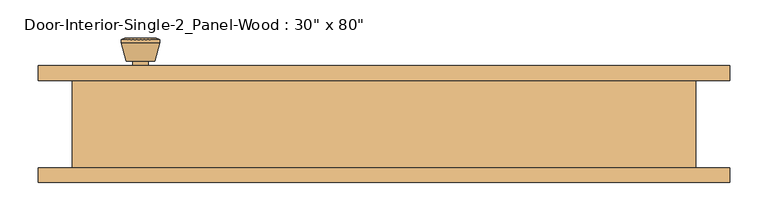
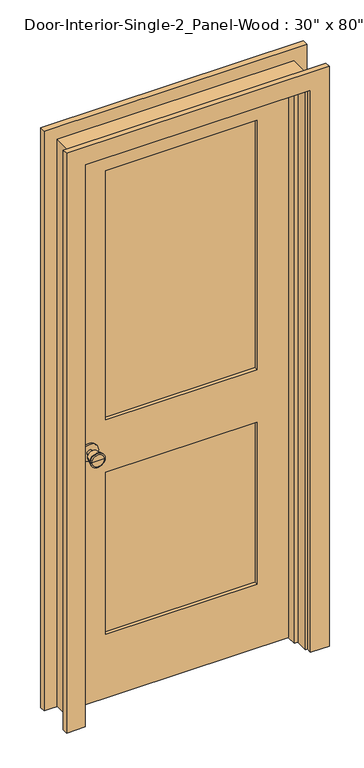
"""IFC4 building model written with IfcOpenShell, lengths in millimetres: door geometry."""

from ifc_helpers import new_model, si_unit, point, frame, frame_2d, origin, place, context, project, spatial, polyline, circle_curve, trimmed, segment, composite_curve, outline, extrude, faceted_brep, source, transform, mapped, element, save
from ifc_brep_helpers import plane_surface, cylinder_surface, revolved_surface, advanced_brep


def door_45c5d68b(model_context):
    return source(origin(), model_context, "Body", "SolidModel", [
        advanced_brep(
        [(-317.5, 13.05, 914.4), (-307.5, 13.05, 914.4), (-327.5, 13.05, 914.4), (-297.0241324, -35.95, 914.4), (-317.5, -35.95, 914.4), (-337.9758676, -35.95, 914.4), (-292.5, -34.1221319, 914.4), (-342.5, -34.1221319, 914.4), (-292.5, -30.6584537, 914.4), (-342.5, -30.6584537, 914.4), (-298.863764, -5.95, 914.4), (-336.136236, -5.95, 914.4), (-307.5, -5.95, 914.4), (-327.5, -5.95, 914.4)],
        [
            (0, 1),
            (1, 2, circle_curve(frame((-317.5, 13.05, 914.4), z_axis=(0.0, 1.0, 0.0), x_axis=(-1.0, 0.0, 0.0)), 10.0)),
            (2, 0),
            (2, 1, circle_curve(frame((-317.5, 13.05, 914.4), z_axis=(0.0, 1.0, 0.0), x_axis=(-1.0, 0.0, 0.0)), 10.0)),
            (3, 4),
            (4, 5),
            (5, 3, circle_curve(frame((-317.5, -35.95, 914.4), z_axis=(0.0, -1.0, 0.0), x_axis=(-1.0, 0.0, 0.0)), 20.4758676)),
            (3, 5, circle_curve(frame((-317.5, -35.95, 914.4), z_axis=(0.0, -1.0, 0.0), x_axis=(-1.0, 0.0, 0.0)), 20.4758676)),
            (6, 3),
            (5, 7),
            (7, 6, circle_curve(frame((-317.5, -34.1221319, 914.4), z_axis=(0.0, -1.0, 0.0), x_axis=(-1.0, 0.0, 0.0)), 25.0)),
            (6, 7, circle_curve(frame((-317.5, -34.1221319, 914.4), z_axis=(0.0, -1.0, 0.0), x_axis=(-1.0, 0.0, 0.0)), 25.0)),
            (8, 6),
            (7, 9),
            (9, 8, circle_curve(frame((-317.5, -30.6584537, 914.4), z_axis=(0.0, -1.0, 0.0), x_axis=(-1.0, 0.0, 0.0)), 25.0)),
            (8, 9, circle_curve(frame((-317.5, -30.6584537, 914.4), z_axis=(0.0, -1.0, 0.0), x_axis=(-1.0, 0.0, 0.0)), 25.0)),
            (10, 8),
            (9, 11),
            (11, 10, circle_curve(frame((-317.5, -5.95, 914.4), z_axis=(0.0, -1.0, 0.0), x_axis=(-1.0, 0.0, 0.0)), 18.636236)),
            (10, 11, circle_curve(frame((-317.5, -5.95, 914.4), z_axis=(0.0, -1.0, 0.0), x_axis=(-1.0, 0.0, 0.0)), 18.636236)),
            (12, 10),
            (11, 13),
            (13, 12, circle_curve(frame((-317.5, -5.95, 914.4), z_axis=(0.0, -1.0, 0.0), x_axis=(-1.0, 0.0, 0.0)), 10.0)),
            (12, 13, circle_curve(frame((-317.5, -5.95, 914.4), z_axis=(0.0, -1.0, 0.0), x_axis=(-1.0, 0.0, 0.0)), 10.0)),
            (1, 12),
            (13, 2),
        ],
        [
            plane_surface(frame((-317.5, 13.05, 914.4), z_axis=(0.0, 1.0, 0.0), x_axis=(-1.0, 0.0, 0.0))),
            plane_surface(frame((-317.5, -35.95, 914.4), z_axis=(0.0, -1.0, 0.0), x_axis=(-1.0, 0.0, 0.0))),
            revolved_surface(polyline([(-337.9758676, -35.95, 914.4), (-342.5, -34.1221319, 914.4)]), (-317.5, 13.05, 914.4), (0.0, 1.0, 0.0)),
            cylinder_surface(frame((-317.5, 13.05, 914.4), z_axis=(0.0, 1.0, 0.0), x_axis=(-1.0, 0.0, 0.0)), 25.0),
            revolved_surface(polyline([(-342.5, -30.6584537, 914.4), (-336.136236, -5.95, 914.4)]), (-317.5, 13.05, 914.4), (0.0, 1.0, 0.0)),
            plane_surface(frame((-317.5, -5.95, 914.4), z_axis=(0.0, 1.0, 0.0), x_axis=(-1.0, 0.0, 0.0))),
            cylinder_surface(frame((-317.5, 13.05, 914.4), z_axis=(0.0, 1.0, 0.0), x_axis=(-1.0, 0.0, 0.0)), 10.0),
        ],
        [
            (0, [[1, 2, 3]]),
            (0, [[-3, 4, -1]]),
            (1, [[5, 6, 7]]),
            (1, [[-6, -5, 8]]),
            (2, [[9, -7, 10, 11]]),
            (2, [[-10, -8, -9, 12]]),
            (3, [[13, -11, 14, 15]]),
            (3, [[-14, -12, -13, 16]]),
            (4, [[17, -15, 18, 19]]),
            (4, [[-18, -16, -17, 20]]),
            (5, [[21, -19, 22, 23]]),
            (5, [[-22, -20, -21, 24]]),
            (6, [[25, -23, 26, -2]]),
            (6, [[-26, -24, -25, -4]]),
        ],
    ),
        extrude(outline(composite_curve([segment(trimmed(circle_curve(frame_2d((914.4, -317.5)), 30.0), [point((914.4, -347.5))], [point((914.4, -287.5))], False, "CARTESIAN"), True, "CONTINUOUS"), segment(trimmed(circle_curve(frame_2d((914.4, -317.5)), 30.0), [point((914.4, -287.5))], [point((914.4, -347.5))], False, "CARTESIAN"), True, "CONTINUOUS")], self_intersect=False)), frame((0.0, 13.05, 0.0), z_axis=(0.0, 1.0, 0.0), x_axis=(0.0, 0.0, 1.0)), (0.0, 0.0, 1.0), 6.0),
        advanced_brep(
        [(-317.5, 59.975, 914.4), (-327.5, 59.975, 914.4), (-307.5, 59.975, 914.4), (-297.0241324, 108.975, 914.4), (-337.9758676, 108.975, 914.4), (-317.5, 108.975, 914.4), (-292.5, 107.1471319, 914.4), (-342.5, 107.1471319, 914.4), (-292.5, 103.6834537, 914.4), (-342.5, 103.6834537, 914.4), (-298.863764, 78.975, 914.4), (-336.136236, 78.975, 914.4), (-307.5, 78.975, 914.4), (-327.5, 78.975, 914.4)],
        [
            (0, 1),
            (1, 2, circle_curve(frame((-317.5, 59.975, 914.4), z_axis=(0.0, -1.0, 0.0), x_axis=(-1.0, 0.0, 0.0)), 10.0)),
            (2, 0),
            (2, 1, circle_curve(frame((-317.5, 59.975, 914.4), z_axis=(0.0, -1.0, 0.0), x_axis=(-1.0, 0.0, 0.0)), 10.0)),
            (3, 4, circle_curve(frame((-317.5, 108.975, 914.4), z_axis=(0.0, 1.0, 0.0), x_axis=(-1.0, 0.0, 0.0)), 20.4758676)),
            (4, 5),
            (5, 3),
            (4, 3, circle_curve(frame((-317.5, 108.975, 914.4), z_axis=(0.0, 1.0, 0.0), x_axis=(-1.0, 0.0, 0.0)), 20.4758676)),
            (6, 7, circle_curve(frame((-317.5, 107.1471319, 914.4), z_axis=(0.0, 1.0, 0.0), x_axis=(-1.0, 0.0, 0.0)), 25.0)),
            (7, 4),
            (3, 6),
            (7, 6, circle_curve(frame((-317.5, 107.1471319, 914.4), z_axis=(0.0, 1.0, 0.0), x_axis=(-1.0, 0.0, 0.0)), 25.0)),
            (8, 9, circle_curve(frame((-317.5, 103.6834537, 914.4), z_axis=(0.0, 1.0, 0.0), x_axis=(-1.0, 0.0, 0.0)), 25.0)),
            (9, 7),
            (6, 8),
            (9, 8, circle_curve(frame((-317.5, 103.6834537, 914.4), z_axis=(0.0, 1.0, 0.0), x_axis=(-1.0, 0.0, 0.0)), 25.0)),
            (10, 11, circle_curve(frame((-317.5, 78.975, 914.4), z_axis=(0.0, 1.0, 0.0), x_axis=(-1.0, 0.0, 0.0)), 18.636236)),
            (11, 9),
            (8, 10),
            (11, 10, circle_curve(frame((-317.5, 78.975, 914.4), z_axis=(0.0, 1.0, 0.0), x_axis=(-1.0, 0.0, 0.0)), 18.636236)),
            (12, 13, circle_curve(frame((-317.5, 78.975, 914.4), z_axis=(0.0, 1.0, 0.0), x_axis=(-1.0, 0.0, 0.0)), 10.0)),
            (13, 11),
            (10, 12),
            (13, 12, circle_curve(frame((-317.5, 78.975, 914.4), z_axis=(0.0, 1.0, 0.0), x_axis=(-1.0, 0.0, 0.0)), 10.0)),
            (1, 13),
            (12, 2),
        ],
        [
            plane_surface(frame((-317.5, 59.975, 914.4), z_axis=(0.0, -1.0, 0.0), x_axis=(-1.0, 0.0, 0.0))),
            plane_surface(frame((-317.5, 108.975, 914.4), z_axis=(0.0, 1.0, 0.0), x_axis=(-1.0, 0.0, 0.0))),
            revolved_surface(polyline([(-337.9758676, 108.975, 914.4), (-342.5, 107.1471319, 914.4)]), (-317.5, 59.975, 914.4), (0.0, -1.0, 0.0)),
            cylinder_surface(frame((-317.5, 59.975, 914.4), z_axis=(0.0, -1.0, 0.0), x_axis=(-1.0, 0.0, 0.0)), 25.0),
            revolved_surface(polyline([(-342.5, 103.6834537, 914.4), (-336.136236, 78.975, 914.4)]), (-317.5, 59.975, 914.4), (0.0, -1.0, 0.0)),
            plane_surface(frame((-317.5, 78.975, 914.4), z_axis=(0.0, -1.0, 0.0), x_axis=(-1.0, 0.0, 0.0))),
            cylinder_surface(frame((-317.5, 59.975, 914.4), z_axis=(0.0, -1.0, 0.0), x_axis=(-1.0, 0.0, 0.0)), 10.0),
        ],
        [
            (0, [[1, 2, 3]]),
            (0, [[-3, 4, -1]]),
            (1, [[5, 6, 7]]),
            (1, [[8, -7, -6]]),
            (2, [[9, 10, -5, 11]]),
            (2, [[12, -11, -8, -10]]),
            (3, [[13, 14, -9, 15]]),
            (3, [[16, -15, -12, -14]]),
            (4, [[17, 18, -13, 19]]),
            (4, [[20, -19, -16, -18]]),
            (5, [[21, 22, -17, 23]]),
            (5, [[24, -23, -20, -22]]),
            (6, [[-2, 25, -21, 26]]),
            (6, [[-4, -26, -24, -25]]),
        ],
    ),
        extrude(outline(composite_curve([segment(trimmed(circle_curve(frame_2d((914.4, -317.5)), 30.0), [point((914.4, -347.5))], [point((914.4, -287.5))], False, "CARTESIAN"), True, "CONTINUOUS"), segment(trimmed(circle_curve(frame_2d((914.4, -317.5)), 30.0), [point((914.4, -287.5))], [point((914.4, -347.5))], False, "CARTESIAN"), True, "CONTINUOUS")], self_intersect=False)), frame((0.0, 53.975, 0.0), z_axis=(0.0, 1.0, 0.0), x_axis=(0.0, 0.0, 1.0)), (0.0, 0.0, 1.0), 6.0),
        faceted_brep([(406.4, 53.975, 0.0), (406.4, -60.325, 0.0), (381.0, -60.325, 0.0), (381.0, -15.875, 0.0), (368.3, -15.875, 0.0), (368.3, 19.05, 0.0), (381.0, 19.05, 0.0), (381.0, 53.975, 0.0), (406.4, 53.975, 2057.4), (406.4, -60.325, 2057.4), (-406.4, -60.325, 2057.4), (-406.4, -60.325, 0.0), (-381.0, -60.325, 0.0), (-381.0, -60.325, 2032.0), (381.0, -60.325, 2032.0), (381.0, -15.875, 2032.0), (-381.0, -15.875, 2032.0), (-381.0, -15.875, 0.0), (-368.3, -15.875, 0.0), (-368.3, -15.875, 2019.3), (368.3, -15.875, 2019.3), (368.3, 19.05, 2019.3), (-368.3, 19.05, 2019.3), (-368.3, 19.05, 0.0), (-381.0, 19.05, 0.0), (-381.0, 19.05, 2032.0), (381.0, 19.05, 2032.0), (381.0, 53.975, 2032.0), (-381.0, 53.975, 2032.0), (-381.0, 53.975, 0.0), (-406.4, 53.975, 0.0), (-406.4, 53.975, 2057.4)], [[[0, 1, 2, 3, 4, 5, 6, 7]], [[1, 0, 8, 9]], [[2, 1, 9, 10, 11, 12, 13, 14]], [[3, 2, 14, 15]], [[4, 3, 15, 16, 17, 18, 19, 20]], [[5, 4, 20, 21]], [[6, 5, 21, 22, 23, 24, 25, 26]], [[7, 6, 26, 27]], [[0, 7, 27, 28, 29, 30, 31, 8]], [[9, 8, 31, 10]], [[15, 14, 13, 16]], [[21, 20, 19, 22]], [[27, 26, 25, 28]], [[30, 29, 24, 23, 18, 17, 12, 11]], [[10, 31, 30, 11]], [[16, 13, 12, 17]], [[22, 19, 18, 23]], [[28, 25, 24, 29]]]),
        extrude(outline(polyline([(2032.0, -381.0), (0.0, -381.0), (0.0, 381.0), (2032.0, 381.0), (2032.0, -381.0)]), holes=[polyline([(1912.9375, -260.35), (1912.9375, 260.35), (1009.65, 260.35), (1009.65, -260.35), (1912.9375, -260.35)]), polyline([(819.15, -260.35), (819.15, 260.35), (231.775, 260.35), (231.775, -260.35), (819.15, -260.35)])]), frame((0.0, 19.05, 0.0), z_axis=(0.0, 1.0, 0.0), x_axis=(0.0, 0.0, 1.0)), (0.0, 0.0, 1.0), 34.925),
        extrude(outline(polyline([(260.35, 30.6916667), (-260.35, 30.6916667), (-260.35, 42.3333333), (260.35, 42.3333333), (260.35, 30.6916667)])), frame((0.0, 0.0, 1009.65), z_axis=(0.0, 0.0, 1.0), x_axis=(1.0, 0.0, 0.0)), (0.0, 0.0, 1.0), 903.2875),
        extrude(outline(polyline([(260.35, 30.6916667), (-260.35, 30.6916667), (-260.35, 42.3333333), (260.35, 42.3333333), (260.35, 30.6916667)])), frame((0.0, 0.0, 231.775), z_axis=(0.0, 0.0, 1.0), x_axis=(1.0, 0.0, 0.0)), (0.0, 0.0, 1.0), 587.375),
        extrude(outline(polyline([(0.0, 387.35), (0.0, 450.85), (2101.85, 450.85), (2101.85, -450.85), (0.0, -450.85), (0.0, -387.35), (2038.35, -387.35), (2038.35, 387.35), (0.0, 387.35)])), frame((0.0, 53.975, 0.0), z_axis=(0.0, 1.0, 0.0), x_axis=(0.0, 0.0, 1.0)), (0.0, 0.0, 1.0), 19.05),
        extrude(outline(polyline([(0.0, 387.35), (0.0, 450.85), (2101.85, 450.85), (2101.85, -450.85), (0.0, -450.85), (0.0, -387.35), (2038.35, -387.35), (2038.35, 387.35), (0.0, 387.35)])), frame((0.0, -79.375, 0.0), z_axis=(0.0, 1.0, 0.0), x_axis=(0.0, 0.0, 1.0)), (0.0, 0.0, 1.0), 19.05),
    ])


if __name__ == "__main__":
    model = new_model("IFC4")
    model_context = context("Model", 3, world=origin())
    ifc_project = project(units=[si_unit("LENGTHUNIT", "METRE", prefix="MILLI")], contexts=[model_context])
    site = spatial("IfcSite", under=ifc_project)
    building = spatial("IfcBuilding", under=site)
    placement = place(None, origin())
    door_shape = door_45c5d68b(model_context)
    element("IfcDoor", 1, ObjectType="Door-Interior-Single-2_Panel-Wood : 30\" x 80\"", at=placement, inside=building, context=model_context, shape_type="MappedRepresentation", body=[
        mapped(door_shape, transform((0.0, 0.0, 0.0), x_axis=(1.0, 0.0, 0.0), y_axis=(0.0, 1.0, 0.0), z_axis=(0.0, 0.0, 1.0))),
    ])
    save(model, "model.ifc")

# Revit data of these elements
# Type "Door-Interior-Single-2_Panel-Wood : 30\" x 80\""
#   Type Mark = "14"
#   Assembly Code = "C1020300"
#   Analytic Construction = "Wooden"
#   Top Rail = 0' - 4 11/16"
#   Thickness = 0' - 1 3/8"
#   Thermal Resistance (R) = 2.5876 (h·ft²·°F)/BTU
#   Swing Angle [instance default] = 90.00°
#   Stiles = 0' - 4 3/4"
#   Rough Width = 2' - 8"
#   Rough Height = 6' - 9"
#   Lock Rail = 0' - 7 1/2"
#   Height = 6' - 8"
#   Width = 2' - 6"
#   Heat Transfer Coefficient (U) = 0.3865 BTU/(h·ft²·°F)
#   Bottom Rail = 0' - 9 1/8"
#   Trim Material = Cherry
#   Panel Material = Cherry
#   Frame Material = Cherry
#   Door Handle Material = Aluminum
#   Visual Light Transmittance = 0
#   Solar Heat Gain Coefficient = 0
#   Wall Closure = (empty or 0)
#   Function = (empty or 0)
# Element 1 (IfcDoor, "Door-Interior-Single-2_Panel-Wood : 30\" x 80\"")
#   Materials on its faces: "Cherry", "Aluminum"
# Materials
#   "Cherry": class "Wood", colour RGB 226 177 128, transparency 0, Description = "Prunus Serotina", Cost = 0
#   "Aluminum": class "Metal", colour RGB 247 247 247, transparency 0, Description = "Aluminum 6061", Cost = 0
